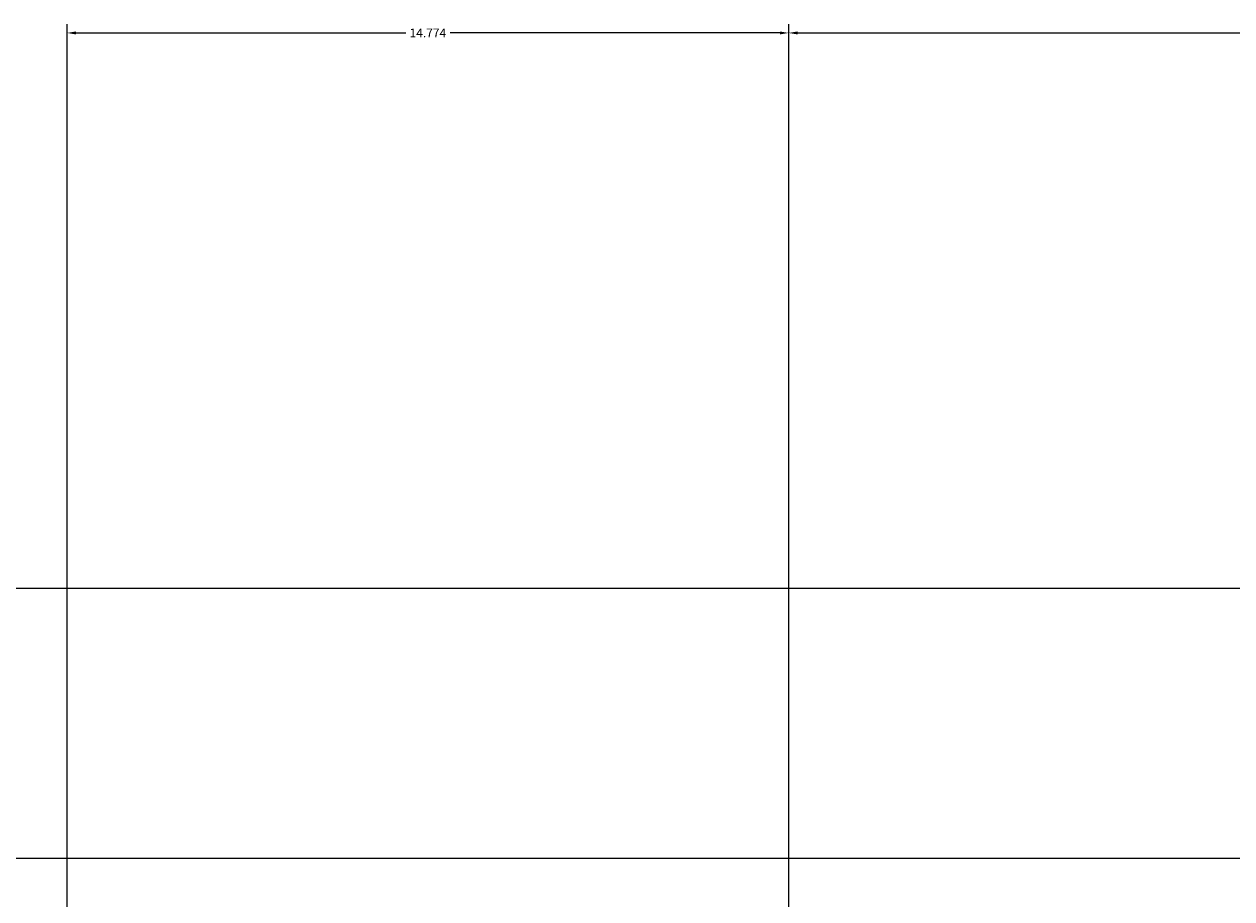
# Model space of a CAD drawing. Units: inches. Extents: x -117 to 121, y -77 to 40.
# Tile 44 of 45: x 72 to 96, y 21 to 39. Entities that reach past the tile are written whole.
import ezdxf

# ---------------------------------------------------------------- set-up
doc = ezdxf.new("R2010")
doc.units = ezdxf.units.IN
doc.header["$MEASUREMENT"] = 0
doc.layers.add('A-ANNO-DIMS', color=2, linetype='Continuous', lineweight=18)
doc.styles.get("Standard").update_dxf_attribs({"font": 'arial.ttf'})
doc.dimstyles.get("Standard").update_dxf_attribs({"dimtxt": 0.18, "dimasz": 0.18, "dimexe": 0.18, "dimexo": 0.0625, "dimgap": 0.09, "dimtad": 0, "dimtih": 1, "dimtoh": 1, "dimdec": 4, "dimzin": 0, "dimdsep": 46, "dimtxsty": 'Standard', "dimcen": 0.09, "dimadec": 0, "dimazin": 0, "dimtfac": 1, "dimtdec": 4, "dimtofl": 0, "dimtmove": 0, "dimatfit": 3, "dimfxl": 1, "dimtolj": 1, "dimtzin": 0, "dimarcsym": 0})

# ---------------------------------------------------------------- blocks, each defined once
blk = doc.blocks.new('*D12')
at = {"layer": 'A-ANNO-DIMS', "color": 0, "lineweight": -2, "transparency": 16777216}
for p, q in [((72.467, -2.59), (72.467, 38.61)), ((87.242, 3.166), (87.242, 38.61)), ((72.647, 38.43), (79.4, 38.43)), ((87.062, 38.43), (80.309, 38.43))]:
    blk.add_line(p, q, dxfattribs=at)
at = {"layer": 'A-ANNO-DIMS', "color": 0, "transparency": 16777216}
for points in [[(72.647, 38.46), (72.647, 38.4), (72.467, 38.43)], [(87.062, 38.46), (87.062, 38.4), (87.242, 38.43)]]:
    blk.add_solid(points, dxfattribs=at)
at = {"layer": 'Defpoints', "color": 0, "transparency": 16777216}
for p in [(87.242, 38.43), (87.242, 3.104), (72.467, -2.653)]:
    blk.add_point(p, dxfattribs=at)
at = {"layer": 'A-ANNO-DIMS', "color": 0, "transparency": 16777216, "insert": (79.854, 38.43), "char_height": 0.18, "attachment_point": 5}
blk.add_mtext('\\A1;14.774', dxfattribs=at)
blk = doc.blocks.new('*D16')
at = {"layer": 'A-ANNO-DIMS', "color": 0, "lineweight": -2, "transparency": 16777216}
for p, q in [((70.862, 21.541), (120.84, 21.541)), ((120.66, 21.361), (120.66, 9.626)), ((120.66, -2.473), (120.66, 9.262)), ((87.304, -2.653), (120.84, -2.653))]:
    blk.add_line(p, q, dxfattribs=at)
at = {"layer": 'A-ANNO-DIMS', "color": 0, "transparency": 16777216}
for points in [[(120.63, 21.361), (120.69, 21.361), (120.66, 21.541)], [(120.63, -2.473), (120.69, -2.473), (120.66, -2.653)]]:
    blk.add_solid(points, dxfattribs=at)
at = {"layer": 'Defpoints', "color": 0, "transparency": 16777216}
for p in [(70.8, 21.541), (87.242, -2.653), (120.66, -2.653)]:
    blk.add_point(p, dxfattribs=at)
at = {"layer": 'A-ANNO-DIMS', "color": 0, "transparency": 16777216, "insert": (120.66, 9.444), "char_height": 0.18, "attachment_point": 5}
blk.add_mtext('\\A1;24.194', dxfattribs=at)
blk = doc.blocks.new('*D17')
at = {"layer": 'A-ANNO-DIMS', "color": 0, "lineweight": -2, "transparency": 16777216}
for p, q in [((14.041, 27.063), (120.84, 27.063)), ((120.66, 26.883), (120.66, 24.484)), ((120.66, 21.721), (120.66, 24.12)), ((70.862, 21.541), (120.84, 21.541))]:
    blk.add_line(p, q, dxfattribs=at)
at = {"layer": 'A-ANNO-DIMS', "color": 0, "transparency": 16777216}
for points in [[(120.63, 26.883), (120.69, 26.883), (120.66, 27.063)], [(120.63, 21.721), (120.69, 21.721), (120.66, 21.541)]]:
    blk.add_solid(points, dxfattribs=at)
at = {"layer": 'Defpoints', "color": 0, "transparency": 16777216}
for p in [(13.978, 27.063), (70.8, 21.541), (120.66, 21.541)]:
    blk.add_point(p, dxfattribs=at)
at = {"layer": 'A-ANNO-DIMS', "color": 0, "transparency": 16777216, "insert": (120.66, 24.302), "char_height": 0.18, "attachment_point": 5}
blk.add_mtext('\\A1;5.522', dxfattribs=at)
blk = doc.blocks.new('*D24')
at = {"layer": 'A-ANNO-DIMS', "color": 0, "lineweight": -2, "transparency": 16777216}
for p, q in [((87.242, 3.166), (87.242, 38.61)), ((109.85, -61.313), (109.85, 38.61)), ((87.422, 38.43), (98.081, 38.43)), ((109.67, 38.43), (99.011, 38.43))]:
    blk.add_line(p, q, dxfattribs=at)
at = {"layer": 'A-ANNO-DIMS', "color": 0, "transparency": 16777216}
for points in [[(87.422, 38.46), (87.422, 38.4), (87.242, 38.43)], [(109.67, 38.46), (109.67, 38.4), (109.85, 38.43)]]:
    blk.add_solid(points, dxfattribs=at)
at = {"layer": 'Defpoints', "color": 0, "transparency": 16777216}
for p in [(109.85, 38.43), (87.242, 3.104), (109.85, -61.376)]:
    blk.add_point(p, dxfattribs=at)
at = {"layer": 'A-ANNO-DIMS', "color": 0, "transparency": 16777216, "insert": (98.546, 38.43), "char_height": 0.18, "attachment_point": 5}
blk.add_mtext('\\A1;22.609', dxfattribs=at)

msp = doc.modelspace()

# ---------------------------------------------------------------- dimensions: what is measured, and where the dimension line sits
at = {"layer": 'A-ANNO-DIMS'}
for base, p1, p2, picture, middle in [((87.241551, 38.429685), (72.467052, -2.65275), (87.241551, 3.103601), '*D12', (79.854301, 38.429685)), ((109.8502, 38.4297), (87.2416, 3.1036), (109.8502, -61.3756), '*D24', (98.5459, 38.4297))]:
    dim = msp.add_linear_dim(base=base, p1=p1, p2=p2, dimstyle='Standard', override={"dimdec": 3, "dimlfac": 1, "dimrnd": 0, "dimzin": 0, "dimdsep": 46, "dimlunit": 2}, dxfattribs=at)
    dim.commit()
    dim.dimension.update_dxf_attribs({"geometry": picture, "text_midpoint": middle})
for base, p1, p2, picture, middle in [((120.6602, 21.5414), (13.9784, 27.0634), (70.8, 21.5414), '*D17', (120.6602, 24.3024)), ((120.6602, -2.6528), (70.8, 21.5414), (87.2416, -2.6528), '*D16', (120.6602, 9.4443))]:
    dim = msp.add_linear_dim(base=base, p1=p1, p2=p2, angle=90, dimstyle='Standard', override={"dimdec": 3, "dimlfac": 1, "dimrnd": 0, "dimzin": 0, "dimdsep": 46, "dimlunit": 2}, dxfattribs=at)
    dim.commit()
    dim.dimension.update_dxf_attribs({"geometry": picture, "text_midpoint": middle})

doc.saveas('drawing.dxf')
